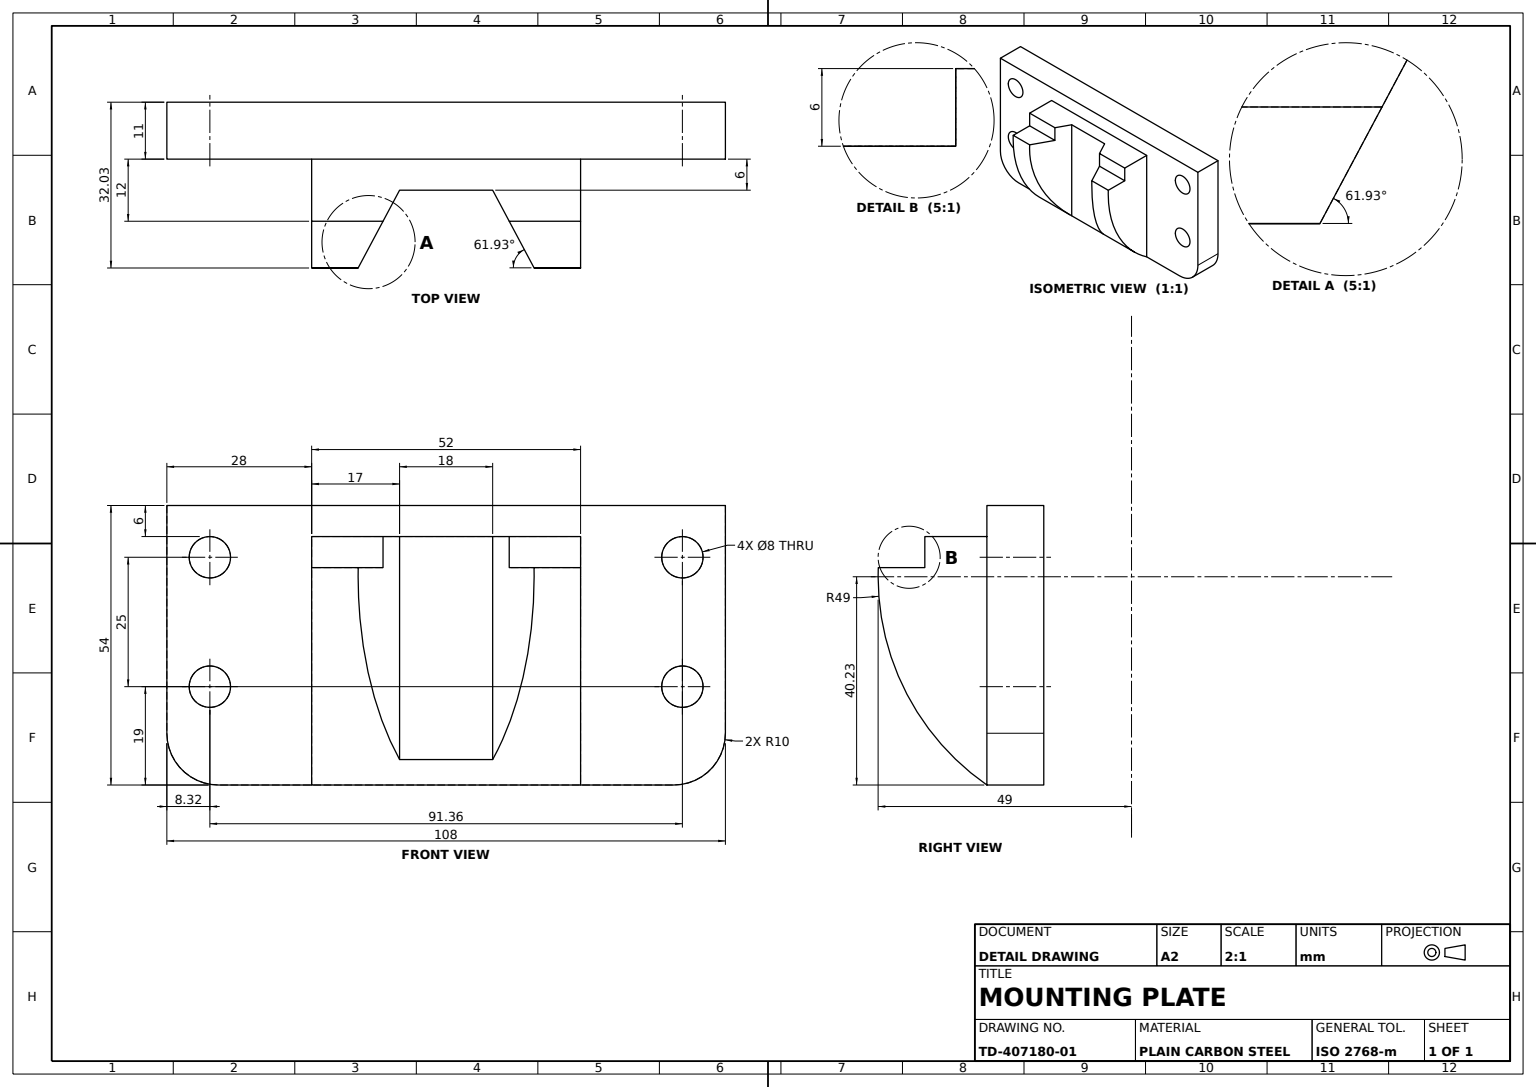
SolidWorks part; units mm, degrees
material "Plain Carbon Steel"
ref_plane "Front Plane" through (0, 0, 0) normal (0, 0, 1) x (1, 0, 0)
ref_plane "Top Plane" through (0, 0, 0) normal (0, 1, 0) x (1, 0, 0)
ref_plane "Right Plane" through (0, 0, 0) normal (1, 0, 0) x (0, 0, -1)
sketch "Base Plate Sketch" plane through (0, 0, 0) normal (0, 0, 1) x (1, 0, 0)
  line L0 (0, 0) -> (0, 59.3543) construction
  line L1 (-54, 27) -> (54, 27)
  line L2 (-54, 27) -> (-54, -17)
  line L3 (-44, -27) -> (44, -27)
  line L4 (54, 27) -> (54, -17)
  line L5 (-54, 27) -> (54, -27) construction
  line L6 (-54, -27) -> (54, 27) construction
  circle A0 centre (-45.6823, 17) radius 4
  circle A1 centre (-45.6823, -8) radius 4
  circle A2 centre (45.6823, -8) radius 4
  circle A3 centre (45.6823, 17) radius 4
  arc A4 (44, -27) -> (54, -17) centre (44, -17) ccw
  arc A5 (-54, -17) -> (-44, -27) centre (-44, -17) ccw
  point P0 (0, 0)
  dimension "D3" = 8
  dimension "D6" = 25
  dimension "D7" = 10
  dimension "D1" = 108
  dimension "D2" = 54
  dimension "D4" = 10
  dimension "D5" = 8.3177
extrude "Base Plate" add sketch "Base Plate Sketch" along normal blind 11
sketch "Guide Block Profile" plane through (0, 0, 0) normal (1, 0, 0) x (0, 0, -1)
  line L0 (-11, 21) -> (-23, 21)
  line L1 (-11, -17) -> (-11, 27) construction
  line L2 (-23, 21) -> (-23, 15)
  line L3 (-23, 15) -> (-32, 15)
  line L4 (-11, 27) -> (0, 27) construction
  line L5 (-11, 21) -> (-11, -27)
  arc A0 (-32, 15) -> (-11, -27) centre (16.9682, 13.2341) ccw
  point P8 (-23, 18)
  dimension "D5" = 49
  dimension "D1" = 6
  dimension "D2" = 12
  dimension "D3" = 21
  dimension "D4" = 6
extrude "Guide Block" add sketch "Guide Block Profile" along normal mid plane 52
sketch "Centre Slot Sketch" plane through (0, 0, 0) normal (0, 1, 0) x (1, 0, 0)
  line L0 (26, -32) -> (-26, -32) construction
  line L1 (-9, -17) -> (-23.3875, -43.9766)
  line L2 (9, -17) -> (23.3875, -43.9766)
  line L3 (-9, -17) -> (9, -17)
  line L5 (54, -11) -> (-54, -11) construction
  line L6 (-23.3875, -43.9766) -> (23.3875, -43.9766)
  circle A0 centre (0, -32) radius 15 construction
  point P8 (0, -17)
  dimension "D1" = 30
  dimension "D2" = 18
  dimension "D3" = 6
  dimension "D4" = 14.3875
extrude "Centre Slot Cut" cut sketch "Centre Slot Sketch" against normal mid plane 52
